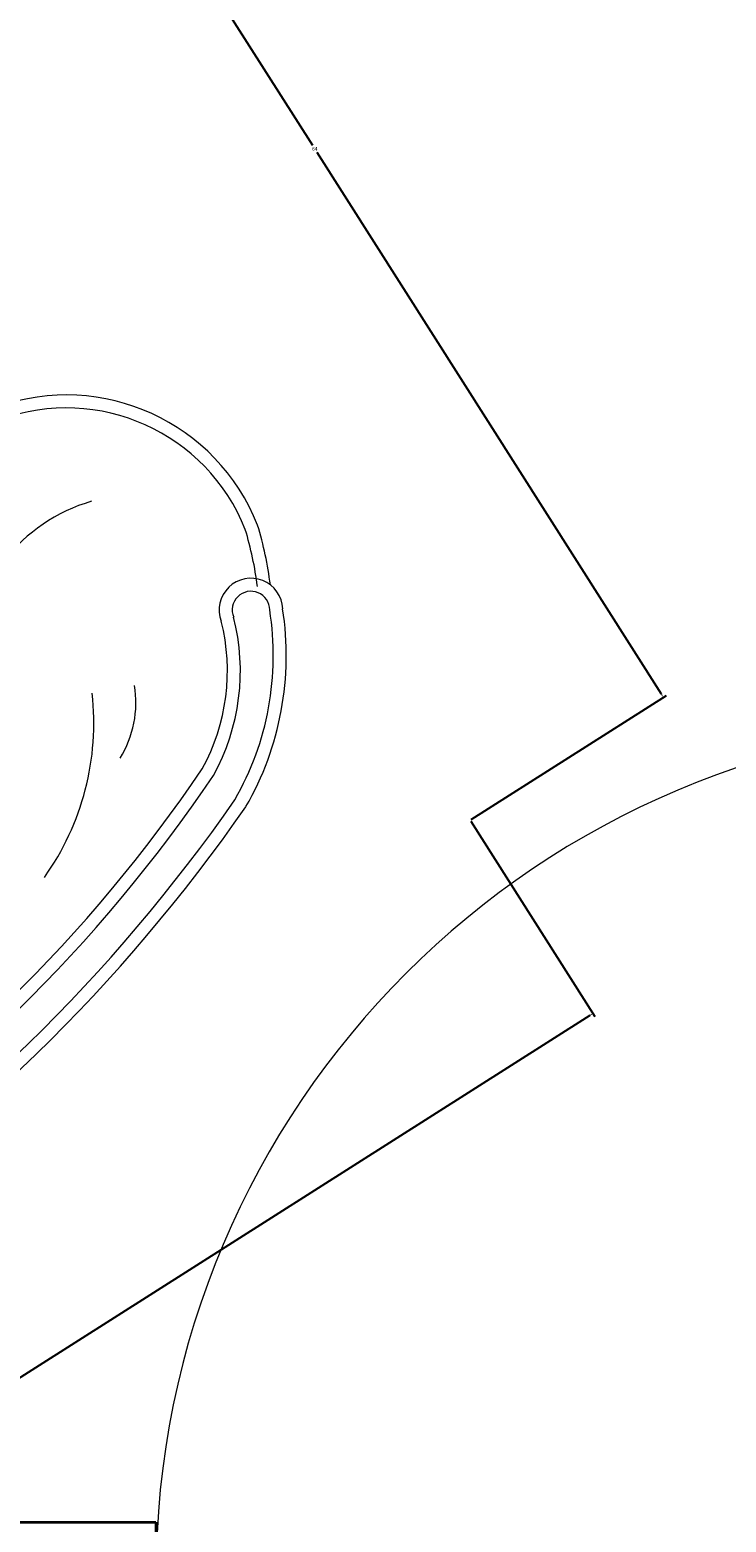
# Model space of a CAD drawing. Units: inches. Extents: x -4843 to -3402, y -164 to 3629.
# Tile 14 of 22: x -4467 to -4433, y 828 to 902. Entities that reach past the tile are written whole.
import ezdxf

# ---------------------------------------------------------------- set-up
doc = ezdxf.new("R2010")
doc.units = ezdxf.units.IN
for name, color, linetype, lineweight in [('A-ANNO-DIMS', 2, 'Continuous', 18), ('doors', 2, 'Continuous', 18), ('furniture', 6, 'Continuous', 18), ('walls', 7, 'Continuous', 35)]:
    doc.layers.add(name, color=color, linetype=linetype, lineweight=lineweight)
doc.styles.get("Standard").update_dxf_attribs({"font": 'arial.ttf'})
doc.dimstyles.get("Standard").update_dxf_attribs({"dimtxt": 0.18, "dimasz": 0.18, "dimexe": 0.18, "dimexo": 0.0625, "dimgap": 0.09, "dimtad": 0, "dimtih": 1, "dimtoh": 1, "dimdec": 4, "dimzin": 0, "dimdsep": 46, "dimtxsty": 'Standard', "dimcen": 0.09, "dimadec": 0, "dimazin": 0, "dimtfac": 1, "dimtdec": 4, "dimtofl": 0, "dimtmove": 0, "dimatfit": 3, "dimfxl": 1, "dimtolj": 1, "dimtzin": 0, "dimarcsym": 0})

# ---------------------------------------------------------------- blocks, each defined once
blk = doc.blocks.new('*U8')
for p, q in [((0, 0), (0, -6)), ((-40, 0), (-40, -6))]:
    blk.add_line(p, q)
blk.add_lwpolyline([(0, 0), (0, 40), (-1.75, 40), (-1.75, 0)], close=True)
blk.add_arc((0, 0), 40, 90, 180)
blk = doc.blocks.new('A$C30AE1D3B')
for centre, radius, start, end in [((1659.5, -897.1, -685.7), 3420.6, 90.7208, 112.8056), ((1659.5, -897.1, -685.7), 3394.2, 90.8361, 112.7864), ((1588.1, -668.8, -685.7), 3092.5, 90.4124, 113.4876), ((1588.1, -668.8, -685.7), 3066.1, 90.5286, 113.4647), ((619.4, 1711.2, -685.7), 615.2, 117.6759, 156.4537), ((619.4, 1711.2, -685.7), 588.8, 117.7842, 156.6248), ((567.5, 1780.8, -685.7), 440.9, 118.7219, 161.8776), ((959.4, 1656.7, -685.7), 540.9, 112.1011, 153.9261), ((567.5, 1780.8, -685.7), 414.5, 118.8865, 161.6537), ((589.4, 1843.7, -685.7), 213.6, 115.7538, 157.0585), ((111, 1924.5, -685.7), 64.4, 149.6532, 348.1693), ((111, 1924.5, -685.7), 38, 147.5708, 350.1051), ((697.5, 1596.6, -685.7), 715.7, 154.6956, 164.5974), ((697.5, 1596.6, -685.7), 689.3, 154.6956, 164.5124), ((416.7, 1707.2, -685.7), 416.9, 169.0069, 345.147), ((416.7, 1707.2, -685.7), 390.5, 169.155, 345.9996), ((363, 1902.3, -685.7), 351.2, 253.9105, 324.4711)]:
    blk.add_arc(centre, radius, start, end)
blk = doc.blocks.new('*D50')
at = {"layer": 'A-ANNO-DIMS', "color": 0, "lineweight": -2, "transparency": 16777216}
for p, q in [((-4445.305, 862.819), (-4439.203, 853.213)), ((-4439.451, 853.269), (-4470.698, 833.416)), ((-4502.521, 813.197), (-4471.274, 833.05)), ((-4508.679, 822.554), (-4502.577, 812.949))]:
    blk.add_line(p, q, dxfattribs=at)
at = {"layer": 'A-ANNO-DIMS', "color": 0, "transparency": 16777216}
for points in [[(-4439.467, 853.294), (-4439.435, 853.243), (-4439.299, 853.365)], [(-4502.537, 813.222), (-4502.505, 813.172), (-4502.673, 813.101)]]:
    blk.add_solid(points, dxfattribs=at)
at = {"layer": 'Defpoints', "color": 0, "transparency": 16777216}
for p in [(-4445.339, 862.871), (-4508.713, 822.607), (-4502.673, 813.101)]:
    blk.add_point(p, dxfattribs=at)
at = {"layer": 'A-ANNO-DIMS', "color": 0, "transparency": 16777216, "insert": (-4470.986, 833.233), "char_height": 0.18, "attachment_point": 5}
blk.add_mtext('\\A1;CHAIR SET 75', dxfattribs=at)
blk = doc.blocks.new('*D51')
at = {"layer": 'A-ANNO-DIMS', "color": 0, "lineweight": -2, "transparency": 16777216}
for p, q in [((-4479.57, 916.866), (-4469.965, 922.969)), ((-4470.021, 922.721), (-4453.091, 896.074)), ((-4435.929, 869.063), (-4452.859, 895.71)), ((-4445.286, 862.905), (-4435.681, 869.008))]:
    blk.add_line(p, q, dxfattribs=at)
at = {"layer": 'A-ANNO-DIMS', "color": 0, "transparency": 16777216}
for points in [[(-4469.995, 922.737), (-4470.046, 922.704), (-4470.117, 922.872)], [(-4435.904, 869.079), (-4435.955, 869.047), (-4435.833, 868.911)]]:
    blk.add_solid(points, dxfattribs=at)
at = {"layer": 'Defpoints', "color": 0, "transparency": 16777216}
for p in [(-4479.623, 916.833), (-4435.833, 868.911), (-4445.339, 862.871)]:
    blk.add_point(p, dxfattribs=at)
at = {"layer": 'A-ANNO-DIMS', "color": 0, "transparency": 16777216, "insert": (-4452.975, 895.892), "char_height": 0.18, "attachment_point": 5}
blk.add_mtext('\\A1;64', dxfattribs=at)

msp = doc.modelspace()

# ---------------------------------------------------------------- linework, layer by layer
at = {"layer": 'walls'}
msp.add_line((-4586.783, 828.354), (-4460.783, 828.354), dxfattribs=at)
msp.add_lwpolyline([(-4460.783, 828.354), (-4460.783, 819.354)], dxfattribs=at)

# ---------------------------------------------------------------- block references
at = {"layer": 'doors', "xscale": 1.05, "yscale": 1.05, "zscale": 1.05}
msp.add_blockref('*U8', (-4418.783, 825.654), dxfattribs=at)
at = {"layer": 'furniture', "xscale": 0.0242257431082848, "yscale": 0.0242257431082848, "zscale": 0.0242257431082848, "rotation": 212.4298414976532}
msp.add_blockref('A$C30AE1D3B', (-4478.842, 914.005, -463.669), dxfattribs=at)

# ---------------------------------------------------------------- dimensions: what is measured, and where the dimension line sits
at = {"layer": 'A-ANNO-DIMS'}
dim = msp.add_linear_dim(base=(-4435.833, 868.911), p1=(-4479.623, 916.833), p2=(-4445.339, 862.871), angle=302.42984, dimstyle='Standard', override={"dimdec": 0, "dimlfac": 1, "dimrnd": 0, "dimzin": 0, "dimdsep": 46, "dimlunit": 2}, dxfattribs=at)
dim.commit()
dim.dimension.update_dxf_attribs({"geometry": '*D51', "text_midpoint": (-4452.975, 895.892)})
dim = msp.add_linear_dim(base=(-4502.673, 813.101), p1=(-4445.339, 862.871), p2=(-4508.713, 822.607), angle=212.42984, text='CHAIR SET <>', dimstyle='Standard', override={"dimdec": 0, "dimlfac": 1, "dimrnd": 0, "dimzin": 0, "dimdsep": 46, "dimlunit": 2}, dxfattribs=at)
dim.commit()
dim.dimension.update_dxf_attribs({"geometry": '*D50', "text_midpoint": (-4470.986, 833.233)})

doc.saveas('drawing.dxf')
